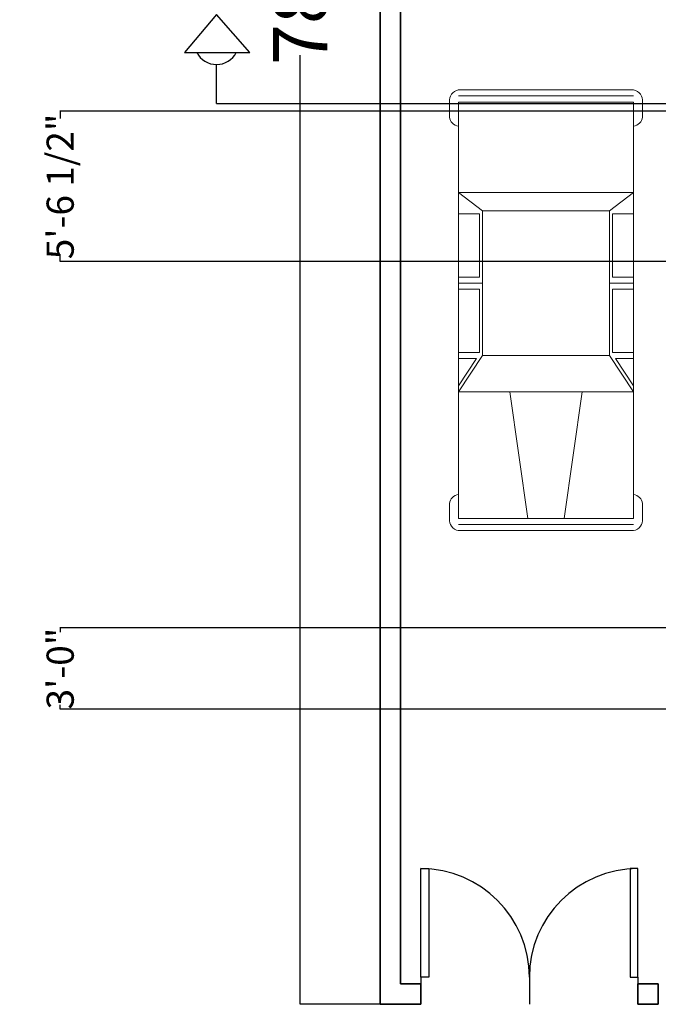
# Model space of a CAD drawing. Units: inches. Extents: x 1146 to 2917, y 889 to 2437.
# Tile 3 of 13: x 1146 to 1428, y 1432 to 1867. Entities that reach past the tile are written whole.
import ezdxf

# ---------------------------------------------------------------- set-up
doc = ezdxf.new("R2010")
doc.units = ezdxf.units.IN
doc.header["$MEASUREMENT"] = 0
for name, color, linetype, lineweight in [('A-ANNO-DIMS', 2, 'Continuous', 18), ('A-ANNO-SYMB', 7, 'Continuous', 25), ('A-SITE-GATE', 10, 'Continuous', 25), ('A-SITE-VEHC', 8, 'Continuous', 13), ('A-SITE-WALL', 7, 'Continuous', 35)]:
    doc.layers.add(name, color=color, linetype=linetype, lineweight=lineweight)
doc.styles.get("Standard").update_dxf_attribs({"font": 'arial.ttf'})
doc.dimstyles.new('Copy of Standard', dxfattribs={"dimtxt": 24, "dimasz": 0.18, "dimexe": 0.18, "dimexo": 0.0625, "dimgap": 0.09, "dimtad": 0, "dimtoh": 1, "dimdec": 1, "dimzin": 0, "dimdsep": 46, "dimlunit": 4, "dimtxsty": 'Standard', "dimcen": 0.09, "dimadec": 0, "dimazin": 0, "dimtfac": 1, "dimtdec": 1, "dimtofl": 0, "dimtmove": 0, "dimatfit": 3, "dimfxl": 1, "dimtolj": 1, "dimtzin": 0, "dimarcsym": 0})
doc.dimstyles.get("Standard").update_dxf_attribs({"dimtxt": 12, "dimasz": 0.18, "dimexe": 0.18, "dimexo": 0.0625, "dimgap": 0.09, "dimtad": 0, "dimtoh": 1, "dimdec": 1, "dimzin": 0, "dimdsep": 46, "dimlunit": 4, "dimtxsty": 'Standard', "dimcen": 0.09, "dimadec": 0, "dimazin": 0, "dimtfac": 1, "dimtdec": 1, "dimtofl": 0, "dimtmove": 0, "dimatfit": 3, "dimfxl": 1, "dimtolj": 1, "dimtzin": 0, "dimarcsym": 0})

# ---------------------------------------------------------------- blocks, each defined once
blk = doc.blocks.new('*U17')
for p, q in [((0, 0), (0, -6)), ((24, 0), (24, -6))]:
    blk.add_line(p, q)
blk.add_lwpolyline([(0, 0), (0, 24), (1.75, 24), (1.75, 0)], close=True)
blk.add_arc((0, 0), 24, 0, 90)
blk = doc.blocks.new('*U18')
for p, q in [((-24, 0), (-24, -6)), ((0, 0), (0, -6))]:
    blk.add_line(p, q)
blk.add_lwpolyline([(0, 0), (0, 24), (-1.75, 24), (-1.75, 0)], close=True)
blk.add_arc((0, 0), 24, 90, 180)
blk = doc.blocks.new('*D54')
at = {"layer": 'A-ANNO-DIMS', "color": 0, "lineweight": -2, "transparency": 16777216}
for p, q in [((1305.07, 2371.39), (1269.65, 2371.39)), ((1269.83, 2371.21), (1269.83, 1951.61)), ((1269.83, 1432.07), (1269.83, 1851.68)), ((1305.07, 1431.89), (1269.65, 1431.89))]:
    blk.add_line(p, q, dxfattribs=at)
at = {"layer": 'A-ANNO-DIMS', "color": 0, "transparency": 16777216}
for points in [[(1269.8, 2371.21), (1269.86, 2371.21), (1269.83, 2371.39)], [(1269.8, 1432.07), (1269.86, 1432.07), (1269.83, 1431.89)]]:
    blk.add_solid(points, dxfattribs=at)
at = {"layer": 'Defpoints', "color": 0, "transparency": 16777216}
for p in [(1305.13, 2371.39), (1269.83, 1431.89), (1305.13, 1431.89)]:
    blk.add_point(p, dxfattribs=at)
at = {"layer": 'A-ANNO-DIMS', "color": 0, "transparency": 16777216, "insert": (1269.83, 1901.64), "char_height": 24, "attachment_point": 5, "rotation": 90}
blk.add_mtext('\\A1;78\'-3{\\H1x;\\S1/2;}"', dxfattribs=at)
blk = doc.blocks.new('*U56')
for p, q in [((5.44, 42.31), (12.12, 42.31)), ((189.69, 42.31), (183.01, 42.31)), ((0.1, -0.41), (0.1, 38.35)), ((2.77, -0.41), (2.77, 38.31)), ((5.44, -0.41), (5.44, 38.24)), ((5.45, 38.31), (16.12, 38.31)), ((16.12, 38.31), (180.34, 38.31)), ((61.52, -0.41), (61.52, 38.31)), ((61.52, 38.31), (77.54, 27.62)), ((64.19, 38.31), (76.2, 30.29)), ((76.2, 30.29), (76.2, 38.31)), ((78.87, 38.31), (78.87, 28.96)), ((106.91, 28.96), (106.91, 38.31)), ((109.58, 27.62), (109.58, 38.31)), ((112.25, 38.31), (112.25, 28.96)), ((140.29, 28.96), (140.29, 38.31)), ((141.62, 27.62), (149.64, 38.31)), ((149.64, -0.41), (149.64, 38.31)), ((189.69, 38.31), (179.01, 38.31)), ((189.69, -0.41), (189.69, 38.24)), ((192.36, -0.41), (192.36, 38.31)), ((195.03, -0.41), (195.03, 38.35)), ((77.54, 27.62), (141.62, 27.62)), ((77.54, -0.41), (77.54, 27.62)), ((78.87, 28.96), (106.91, 28.96)), ((112.25, 28.96), (140.29, 28.96)), ((141.62, -0.41), (141.62, 27.62)), ((5.44, 7.6), (61.52, 15.61)), ((0.1, -0.42), (0.1, -39.18)), ((2.77, -0.41), (2.77, -39.13)), ((5.44, -0.42), (5.44, -39.07)), ((61.52, -0.41), (61.52, -39.13)), ((77.54, -0.41), (77.54, -28.45)), ((141.62, -0.41), (141.62, -28.45)), ((149.64, -0.41), (149.64, -39.13)), ((189.69, -0.42), (189.69, -39.07)), ((192.36, -0.41), (192.36, -39.13)), ((195.03, -0.42), (195.03, -39.18)), ((5.44, -8.42), (61.52, -16.43)), ((61.52, -39.13), (77.54, -28.45)), ((77.54, -28.45), (141.62, -28.45)), ((78.87, -39.13), (78.87, -29.79)), ((78.87, -29.79), (106.91, -29.79)), ((106.91, -29.79), (106.91, -39.13)), ((109.58, -28.45), (109.58, -39.13)), ((112.25, -29.79), (140.29, -29.79)), ((112.25, -39.13), (112.25, -29.79)), ((140.29, -29.79), (140.29, -39.13)), ((141.62, -28.45), (149.64, -39.13)), ((64.19, -39.13), (76.2, -31.12)), ((76.2, -31.12), (76.2, -39.13)), ((5.45, -39.13), (16.12, -39.13)), ((16.12, -39.13), (180.34, -39.13)), ((189.69, -39.13), (179.01, -39.13)), ((5.44, -43.14), (12.12, -43.14)), ((189.69, -43.14), (183.01, -43.14))]:
    blk.add_line(p, q)
for centre, radius, start, end in [((5.06, 37.26), 5.06, 85.6455, 168.0943), ((11.45, 37.64), 4.72, 8.1301, 81.87), ((183.68, 37.64), 4.72, 98.13, 171.8699), ((190.07, 37.26), 5.06, 11.9057, 94.3545), ((5.06, -38.09), 5.06, 191.9057, 274.3545), ((11.45, -38.46), 4.72, 278.13, 351.8699), ((183.68, -38.46), 4.72, 188.1301, 261.87), ((190.07, -38.09), 5.06, 265.6455, 348.0943)]:
    blk.add_arc(centre, radius, start, end)
blk = doc.blocks.new('SECTION-HEAD')
for p, q in [((14.15, 39.3), (0, 22.6)), ((28.83, 22.6), (14.15, 39.3)), ((0, 22.6), (28.83, 22.6)), ((14.15, 0), (14.15, 17.21))]:
    blk.add_line(p, q)
blk.add_arc((14.15, 26.98), 9.77, 206.6471, 333.3529)
blk = doc.blocks.new('*D170')
at = {"layer": 'A-ANNO-DIMS', "color": 0, "lineweight": -2, "transparency": 16777216}
for p, q in [((1461.07, 1598.39), (1163.51, 1598.39)), ((1163.69, 1598.21), (1163.69, 1596.43)), ((1163.69, 1562.57), (1163.69, 1564.36)), ((1461.07, 1562.39), (1163.51, 1562.39))]:
    blk.add_line(p, q, dxfattribs=at)
at = {"layer": 'A-ANNO-DIMS', "color": 0, "transparency": 16777216}
for points in [[(1163.66, 1598.21), (1163.72, 1598.21), (1163.69, 1598.39)], [(1163.66, 1562.57), (1163.72, 1562.57), (1163.69, 1562.39)]]:
    blk.add_solid(points, dxfattribs=at)
at = {"layer": 'Defpoints', "color": 0, "transparency": 16777216}
for p in [(1461.13, 1598.39), (1163.69, 1562.39), (1461.13, 1562.39)]:
    blk.add_point(p, dxfattribs=at)
at = {"layer": 'A-ANNO-DIMS', "color": 0, "transparency": 16777216, "insert": (1163.69, 1580.39), "char_height": 12, "attachment_point": 5, "rotation": 90}
blk.add_mtext('\\A1;3\'-0"', dxfattribs=at)
blk = doc.blocks.new('*D171')
at = {"layer": 'A-ANNO-DIMS', "color": 0, "lineweight": -2, "transparency": 16777216}
for p, q in [((1549.57, 1826.89), (1163.51, 1826.89)), ((1163.69, 1826.71), (1163.69, 1823.66)), ((1545.07, 1760.39), (1163.51, 1760.39)), ((1163.69, 1760.57), (1163.69, 1763.62))]:
    blk.add_line(p, q, dxfattribs=at)
at = {"layer": 'A-ANNO-DIMS', "color": 0, "transparency": 16777216}
for points in [[(1163.66, 1826.71), (1163.72, 1826.71), (1163.69, 1826.89)], [(1163.66, 1760.57), (1163.72, 1760.57), (1163.69, 1760.39)]]:
    blk.add_solid(points, dxfattribs=at)
at = {"layer": 'Defpoints', "color": 0, "transparency": 16777216}
for p in [(1549.63, 1826.89), (1163.69, 1760.39), (1545.13, 1760.39)]:
    blk.add_point(p, dxfattribs=at)
at = {"layer": 'A-ANNO-DIMS', "color": 0, "transparency": 16777216, "insert": (1163.69, 1793.64), "char_height": 12, "attachment_point": 5, "rotation": 90}
blk.add_mtext('\\A1;5\'-6 1/2"', dxfattribs=at)

msp = doc.modelspace()

# ---------------------------------------------------------------- linework, layer by layer
at = {"layer": 'A-ANNO-SYMB'}
msp.add_line((1232.84, 1830.35), (2074.15, 1830.35), dxfattribs=at)
at = {"layer": 'A-SITE-WALL'}
for p, q in [((1305.13, 2254.39), (1305.13, 1431.89)), ((1314.13, 2254.39), (1314.13, 1440.89)), ((1314.13, 1440.89), (1323.13, 1440.89)), ((1323.13, 1440.89), (1323.13, 1431.89)), ((1419.13, 1440.89), (1419.13, 1431.89)), ((1419.13, 1440.89), (1428.13, 1440.89)), ((1428.13, 1440.89), (1428.13, 1431.89)), ((1305.13, 1431.89), (1323.13, 1431.89)), ((1419.13, 1431.89), (1428.13, 1431.89))]:
    msp.add_line(p, q, dxfattribs=at)

# ---------------------------------------------------------------- block references
at = {"layer": 'A-ANNO-SYMB'}
msp.add_blockref('SECTION-HEAD', (1218.69, 1830.35), dxfattribs=at)
at = {"layer": 'A-SITE-GATE', "xscale": 2, "yscale": 2, "zscale": 2}
for name, p in [('*U17', (1323.13, 1443.89)), ('*U18', (1419.13, 1443.89))]:
    msp.add_blockref(name, p, dxfattribs=at)
at = {"layer": 'A-SITE-VEHC', "rotation": 90}
msp.add_blockref('*U56', (1378.06, 1641.29), dxfattribs=at)

# ---------------------------------------------------------------- dimensions: what is measured, and where the dimension line sits
at = {"layer": 'A-ANNO-DIMS'}
dim = msp.add_linear_dim(base=(1269.83, 1431.89), p1=(1305.13, 2371.39), p2=(1305.13, 1431.89), angle=270, dimstyle='Copy of Standard', override={"dimclrd": 0, "dimclre": 0, "dimclrt": 0}, dxfattribs=at)
dim.commit()
dim.dimension.update_dxf_attribs({"geometry": '*D54', "text_midpoint": (1269.83, 1901.64), "dimtype": 161})
for base, p1, p2, picture, middle in [((1163.69, 1760.39), (1549.63, 1826.89), (1545.13, 1760.39), '*D171', (1163.69, 1793.64)), ((1163.69, 1562.39), (1461.13, 1598.39), (1461.13, 1562.39), '*D170', (1163.69, 1580.39))]:
    dim = msp.add_linear_dim(base=base, p1=p1, p2=p2, angle=90, dimstyle='Standard', override={"dimdec": 1, "dimlfac": 1, "dimrnd": 0, "dimzin": 1, "dimdsep": 46, "dimlunit": 4, "dimfrac": 2}, dxfattribs=at)
    dim.commit()
    dim.dimension.update_dxf_attribs({"geometry": picture, "text_midpoint": middle})

doc.saveas('drawing.dxf')
